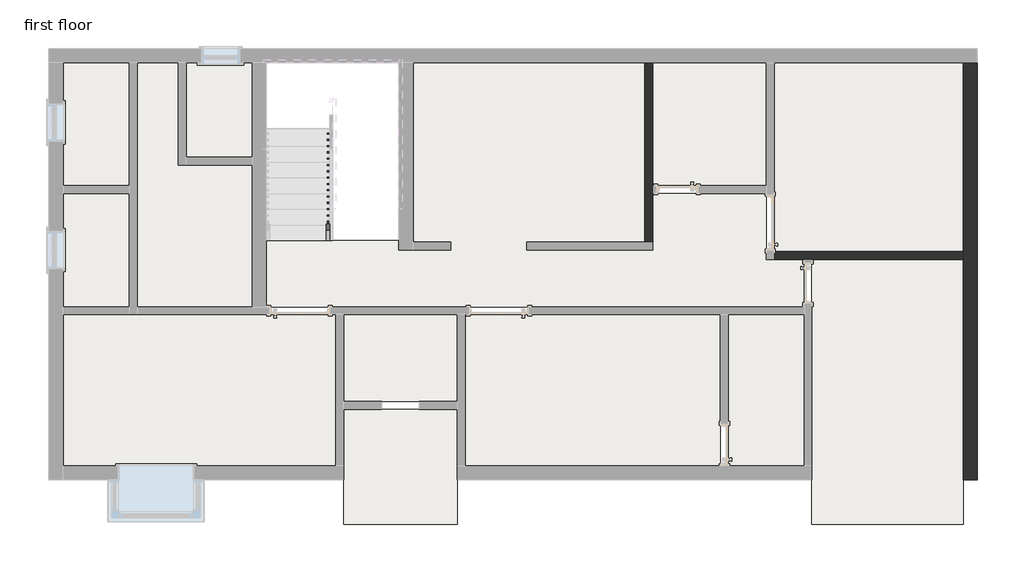
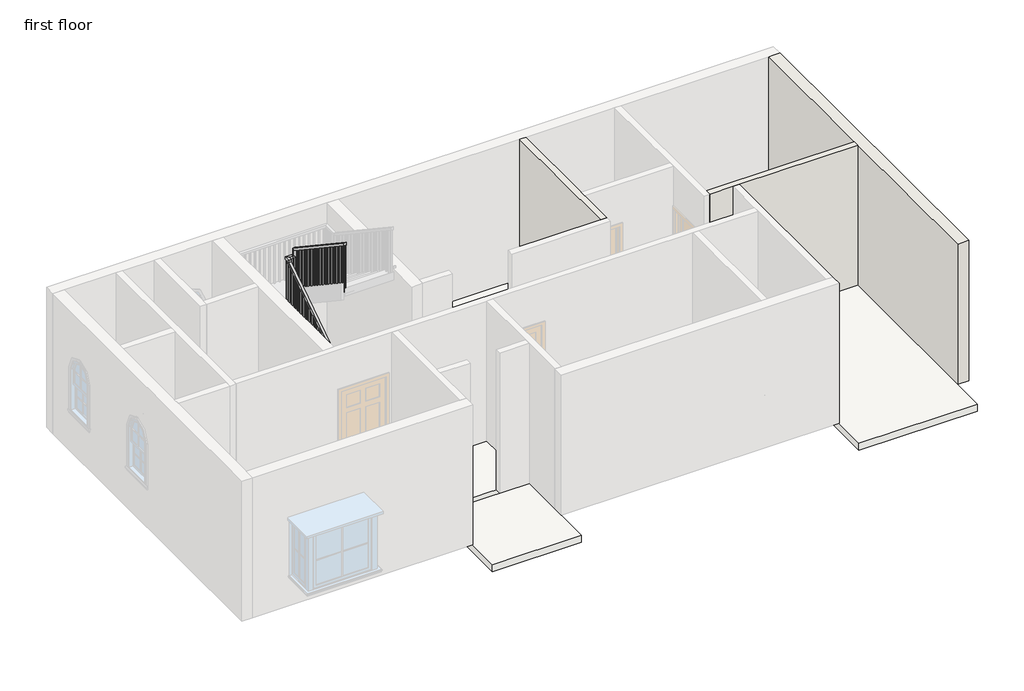
# One storey, part 2 of 3: 3 walls, 2 slabs, 1 railing.
"""IFC4 building model written with IfcOpenShell, lengths in millimetres."""

from ifc_helpers import new_model, si_unit, frame, origin, place, context, project, spatial, polyline, outline, extrude, faceted_brep, element, save

model = new_model("IFC4")

# Units and contexts
model_context = context("Model", 3, world=origin())
ifc_project = project(units=[si_unit("LENGTHUNIT", "METRE", prefix="MILLI")], contexts=[model_context])

# Site, building, storey
site = spatial("IfcSite", under=ifc_project)
building = spatial("IfcBuilding", under=site)
storey = spatial("IfcBuildingStorey", under=building, Name="first floor", Elevation=3352.8)

# Railing
placement = place(None, origin())
element("IfcRailing", 1, ObjectType="Handrail - Rectangular", at=placement, inside=storey, context=model_context, shape_type="SolidModel", body=[
    faceted_brep([(-8708.6672301, -3404.4302427, 4436.5333333), (-8708.6672301, -3404.4302427, 4375.4793317), (-8657.8672301, -3404.4302427, 4375.4793317), (-8657.8672301, -3404.4302427, 4436.5333333), (-8708.6672301, -1194.6302427, 5909.7333333), (-8708.6672301, -1143.8302427, 5882.5459984), (-8657.8672301, -1143.8302427, 5882.5459984), (-8657.8672301, -1194.6302427, 5909.7333333), (-8708.6672301, -1194.6302427, 5960.5333333), (-8708.6672301, -1143.8302427, 5909.7333333), (-8657.8672301, -1143.8302427, 5909.7333333), (-8657.8672301, -1194.6302427, 5960.5333333), (-8708.6672301, -1067.6302427, 5960.5333333), (-8708.6672301, -1067.6302427, 5909.7333333), (-8657.8672301, -1118.4302427, 5909.7333333), (-8657.8672301, -1118.4302427, 5960.5333333), (-8581.6672301, -1067.6302427, 5960.5333333), (-8581.6672301, -1067.6302427, 5909.7333333), (-8581.6672301, -1118.4302427, 5909.7333333), (-8581.6672301, -1118.4302427, 5960.5333333), (-8556.2672301, -1067.6302427, 5960.5333333), (-8556.2672301, -1118.4302427, 5960.5333333), (-8505.4672301, -1118.4302427, 5909.7333333), (-8505.4672301, -1067.6302427, 5909.7333333)], [[[0, 1, 2, 3]], [[1, 0, 4, 5]], [[2, 1, 5, 6]], [[3, 2, 6, 7]], [[0, 3, 7, 4]], [[5, 4, 8, 9]], [[6, 5, 9, 10]], [[7, 6, 10, 11]], [[4, 7, 11, 8]], [[9, 8, 12, 13]], [[10, 9, 13, 14]], [[11, 10, 14, 15]], [[8, 11, 15, 12]], [[13, 12, 16, 17]], [[14, 13, 17, 18]], [[15, 14, 18, 19]], [[12, 15, 19, 16]], [[20, 21, 22, 23]], [[17, 16, 20, 23]], [[18, 17, 23, 22]], [[19, 18, 22, 21]], [[16, 19, 21, 20]]]),
    faceted_brep([(-8556.2672301, -1067.6302427, 5960.5333333), (-8505.4672301, -1067.6302427, 5909.7333333), (-8505.4672301, -1118.4302427, 5909.7333333), (-8556.2672301, -1118.4302427, 5960.5333333), (-8556.2672301, -1067.6302427, 6096.0), (-8556.2672301, -1118.4302427, 6068.8126651), (-8505.4672301, -1118.4302427, 6068.8126651), (-8505.4672301, -1067.6302427, 6096.0)], [[[0, 1, 2, 3]], [[4, 5, 6, 7]], [[1, 0, 4, 7]], [[2, 1, 7, 6]], [[3, 2, 6, 5]], [[0, 3, 5, 4]]]),
    faceted_brep([(-8505.4672301, -1067.6302427, 6096.0), (-8505.4672301, -1118.4302427, 6068.8126651), (-8556.2672301, -1118.4302427, 6068.8126651), (-8556.2672301, -1067.6302427, 6096.0), (-8505.4672301, -2896.4302427, 7315.2), (-8556.2672301, -2896.4302427, 7315.2), (-8556.2672301, -2896.4302427, 7254.1459984), (-8505.4672301, -2896.4302427, 7254.1459984)], [[[0, 1, 2, 3]], [[4, 5, 6, 7]], [[1, 0, 4, 7]], [[2, 1, 7, 6]], [[3, 2, 6, 5]], [[0, 3, 5, 4]]]),
    extrude(outline(polyline([(-2829.7552427, 7209.6959984), (-2810.7052427, 7196.9959984), (-2810.7052427, 6231.4666667), (-2829.7552427, 6231.4666667), (-2829.7552427, 7209.6959984)])), frame((-8540.3922301, 0.0, 0.0), z_axis=(1.0, 0.0, 0.0), x_axis=(0.0, 1.0, 0.0)), (0.0, 0.0, 1.0), 19.05),
    extrude(outline(polyline([(-2728.1552427, 7141.9626651), (-2709.1052427, 7129.2626651), (-2709.1052427, 6231.4666667), (-2728.1552427, 6231.4666667), (-2728.1552427, 7141.9626651)])), frame((-8540.3922301, 0.0, 0.0), z_axis=(1.0, 0.0, 0.0), x_axis=(0.0, 1.0, 0.0)), (0.0, 0.0, 1.0), 19.05),
    extrude(outline(polyline([(-2626.5552427, 7074.2293317), (-2607.5052427, 7061.5293317), (-2607.5052427, 6062.1333333), (-2626.5552427, 6062.1333333), (-2626.5552427, 7074.2293317)])), frame((-8540.3922301, 0.0, 0.0), z_axis=(1.0, 0.0, 0.0), x_axis=(0.0, 1.0, 0.0)), (0.0, 0.0, 1.0), 19.05),
    extrude(outline(polyline([(-2524.9552427, 7006.4959984), (-2505.9052427, 6993.7959984), (-2505.9052427, 6062.1333333), (-2524.9552427, 6062.1333333), (-2524.9552427, 7006.4959984)])), frame((-8540.3922301, 0.0, 0.0), z_axis=(1.0, 0.0, 0.0), x_axis=(0.0, 1.0, 0.0)), (0.0, 0.0, 1.0), 19.05),
    extrude(outline(polyline([(-2423.3552427, 6938.7626651), (-2404.3052427, 6926.0626651), (-2404.3052427, 6062.1333333), (-2423.3552427, 6062.1333333), (-2423.3552427, 6938.7626651)])), frame((-8540.3922301, 0.0, 0.0), z_axis=(1.0, 0.0, 0.0), x_axis=(0.0, 1.0, 0.0)), (0.0, 0.0, 1.0), 19.05),
    extrude(outline(polyline([(-2321.7552427, 6871.0293317), (-2302.7052427, 6858.3293317), (-2302.7052427, 5892.8), (-2321.7552427, 5892.8), (-2321.7552427, 6871.0293317)])), frame((-8540.3922301, 0.0, 0.0), z_axis=(1.0, 0.0, 0.0), x_axis=(0.0, 1.0, 0.0)), (0.0, 0.0, 1.0), 19.05),
    extrude(outline(polyline([(-2220.1552427, 6803.2959984), (-2201.1052427, 6790.5959984), (-2201.1052427, 5892.8), (-2220.1552427, 5892.8), (-2220.1552427, 6803.2959984)])), frame((-8540.3922301, 0.0, 0.0), z_axis=(1.0, 0.0, 0.0), x_axis=(0.0, 1.0, 0.0)), (0.0, 0.0, 1.0), 19.05),
    extrude(outline(polyline([(-2118.5552427, 6735.5626651), (-2099.5052427, 6722.8626651), (-2099.5052427, 5723.4666667), (-2118.5552427, 5723.4666667), (-2118.5552427, 6735.5626651)])), frame((-8540.3922301, 0.0, 0.0), z_axis=(1.0, 0.0, 0.0), x_axis=(0.0, 1.0, 0.0)), (0.0, 0.0, 1.0), 19.05),
    extrude(outline(polyline([(-2016.9552427, 6667.8293317), (-1997.9052427, 6655.1293317), (-1997.9052427, 5723.4666667), (-2016.9552427, 5723.4666667), (-2016.9552427, 6667.8293317)])), frame((-8540.3922301, 0.0, 0.0), z_axis=(1.0, 0.0, 0.0), x_axis=(0.0, 1.0, 0.0)), (0.0, 0.0, 1.0), 19.05),
    extrude(outline(polyline([(-1915.3552427, 6600.0959984), (-1896.3052427, 6587.3959984), (-1896.3052427, 5723.4666667), (-1915.3552427, 5723.4666667), (-1915.3552427, 6600.0959984)])), frame((-8540.3922301, 0.0, 0.0), z_axis=(1.0, 0.0, 0.0), x_axis=(0.0, 1.0, 0.0)), (0.0, 0.0, 1.0), 19.05),
    extrude(outline(polyline([(-1813.7552427, 6532.3626651), (-1794.7052427, 6519.6626651), (-1794.7052427, 5554.1333333), (-1813.7552427, 5554.1333333), (-1813.7552427, 6532.3626651)])), frame((-8540.3922301, 0.0, 0.0), z_axis=(1.0, 0.0, 0.0), x_axis=(0.0, 1.0, 0.0)), (0.0, 0.0, 1.0), 19.05),
    extrude(outline(polyline([(-1712.1552427, 6464.6293317), (-1693.1052427, 6451.9293317), (-1693.1052427, 5554.1333333), (-1712.1552427, 5554.1333333), (-1712.1552427, 6464.6293317)])), frame((-8540.3922301, 0.0, 0.0), z_axis=(1.0, 0.0, 0.0), x_axis=(0.0, 1.0, 0.0)), (0.0, 0.0, 1.0), 19.05),
    extrude(outline(polyline([(-1610.5552427, 6396.8959984), (-1591.5052427, 6384.1959984), (-1591.5052427, 5384.8), (-1610.5552427, 5384.8), (-1610.5552427, 6396.8959984)])), frame((-8540.3922301, 0.0, 0.0), z_axis=(1.0, 0.0, 0.0), x_axis=(0.0, 1.0, 0.0)), (0.0, 0.0, 1.0), 19.05),
    extrude(outline(polyline([(-1508.9552427, 6329.1626651), (-1489.9052427, 6316.4626651), (-1489.9052427, 5384.8), (-1508.9552427, 5384.8), (-1508.9552427, 6329.1626651)])), frame((-8540.3922301, 0.0, 0.0), z_axis=(1.0, 0.0, 0.0), x_axis=(0.0, 1.0, 0.0)), (0.0, 0.0, 1.0), 19.05),
    extrude(outline(polyline([(-1407.3552427, 6261.4293317), (-1388.3052427, 6248.7293317), (-1388.3052427, 5384.8), (-1407.3552427, 5384.8), (-1407.3552427, 6261.4293317)])), frame((-8540.3922301, 0.0, 0.0), z_axis=(1.0, 0.0, 0.0), x_axis=(0.0, 1.0, 0.0)), (0.0, 0.0, 1.0), 19.05),
    extrude(outline(polyline([(-1305.7552427, 6193.6959984), (-1286.7052427, 6180.9959984), (-1286.7052427, 5215.4666667), (-1305.7552427, 5215.4666667), (-1305.7552427, 6193.6959984)])), frame((-8540.3922301, 0.0, 0.0), z_axis=(1.0, 0.0, 0.0), x_axis=(0.0, 1.0, 0.0)), (0.0, 0.0, 1.0), 19.05),
    extrude(outline(polyline([(-1204.1552427, 6125.9626651), (-1185.1052427, 6113.2626651), (-1185.1052427, 5215.4666667), (-1204.1552427, 5215.4666667), (-1204.1552427, 6125.9626651)])), frame((-8540.3922301, 0.0, 0.0), z_axis=(1.0, 0.0, 0.0), x_axis=(0.0, 1.0, 0.0)), (0.0, 0.0, 1.0), 19.05),
    extrude(outline(polyline([(-8591.1922301, -1102.5552427), (-8591.1922301, -1083.5052427), (-8572.1422301, -1083.5052427), (-8572.1422301, -1102.5552427), (-8591.1922301, -1102.5552427)])), frame((0.0, 0.0, 5046.1333333), z_axis=(0.0, 0.0, 1.0), x_axis=(1.0, 0.0, 0.0)), (0.0, 0.0, 1.0), 863.6),
    extrude(outline(polyline([(-8673.7422301, -1178.7552427), (-8692.7922301, -1178.7552427), (-8692.7922301, -1159.7052427), (-8673.7422301, -1159.7052427), (-8673.7422301, -1178.7552427)])), frame((0.0, 0.0, 4876.8), z_axis=(0.0, 0.0, 1.0), x_axis=(1.0, 0.0, 0.0)), (0.0, 0.0, 1.0), 1032.9333333),
    extrude(outline(polyline([(-1280.3552427, 5791.5293317), (-1261.3052427, 5804.2293317), (-1261.3052427, 4876.8), (-1280.3552427, 4876.8), (-1280.3552427, 5791.5293317)])), frame((-8692.7922301, 0.0, 0.0), z_axis=(1.0, 0.0, 0.0), x_axis=(0.0, 1.0, 0.0)), (0.0, 0.0, 1.0), 19.05),
    extrude(outline(polyline([(-1381.9552427, 5723.7959984), (-1362.9052427, 5736.4959984), (-1362.9052427, 4876.8), (-1381.9552427, 4876.8), (-1381.9552427, 5723.7959984)])), frame((-8692.7922301, 0.0, 0.0), z_axis=(1.0, 0.0, 0.0), x_axis=(0.0, 1.0, 0.0)), (0.0, 0.0, 1.0), 19.05),
    extrude(outline(polyline([(-1483.5552427, 5656.0626651), (-1464.5052427, 5668.7626651), (-1464.5052427, 4707.4666667), (-1483.5552427, 4707.4666667), (-1483.5552427, 5656.0626651)])), frame((-8692.7922301, 0.0, 0.0), z_axis=(1.0, 0.0, 0.0), x_axis=(0.0, 1.0, 0.0)), (0.0, 0.0, 1.0), 19.05),
    extrude(outline(polyline([(-1585.1552427, 5588.3293317), (-1566.1052427, 5601.0293317), (-1566.1052427, 4707.4666667), (-1585.1552427, 4707.4666667), (-1585.1552427, 5588.3293317)])), frame((-8692.7922301, 0.0, 0.0), z_axis=(1.0, 0.0, 0.0), x_axis=(0.0, 1.0, 0.0)), (0.0, 0.0, 1.0), 19.05),
    extrude(outline(polyline([(-1686.7552427, 5520.5959984), (-1667.7052427, 5533.2959984), (-1667.7052427, 4538.1333333), (-1686.7552427, 4538.1333333), (-1686.7552427, 5520.5959984)])), frame((-8692.7922301, 0.0, 0.0), z_axis=(1.0, 0.0, 0.0), x_axis=(0.0, 1.0, 0.0)), (0.0, 0.0, 1.0), 19.05),
    extrude(outline(polyline([(-1788.3552427, 5452.8626651), (-1769.3052427, 5465.5626651), (-1769.3052427, 4538.1333333), (-1788.3552427, 4538.1333333), (-1788.3552427, 5452.8626651)])), frame((-8692.7922301, 0.0, 0.0), z_axis=(1.0, 0.0, 0.0), x_axis=(0.0, 1.0, 0.0)), (0.0, 0.0, 1.0), 19.05),
    extrude(outline(polyline([(-1889.9552427, 5385.1293317), (-1870.9052427, 5397.8293317), (-1870.9052427, 4538.1333333), (-1889.9552427, 4538.1333333), (-1889.9552427, 5385.1293317)])), frame((-8692.7922301, 0.0, 0.0), z_axis=(1.0, 0.0, 0.0), x_axis=(0.0, 1.0, 0.0)), (0.0, 0.0, 1.0), 19.05),
    extrude(outline(polyline([(-1991.5552427, 5317.3959984), (-1972.5052427, 5330.0959984), (-1972.5052427, 4368.8), (-1991.5552427, 4368.8), (-1991.5552427, 5317.3959984)])), frame((-8692.7922301, 0.0, 0.0), z_axis=(1.0, 0.0, 0.0), x_axis=(0.0, 1.0, 0.0)), (0.0, 0.0, 1.0), 19.05),
    extrude(outline(polyline([(-2093.1552427, 5249.6626651), (-2074.1052427, 5262.3626651), (-2074.1052427, 4368.8), (-2093.1552427, 4368.8), (-2093.1552427, 5249.6626651)])), frame((-8692.7922301, 0.0, 0.0), z_axis=(1.0, 0.0, 0.0), x_axis=(0.0, 1.0, 0.0)), (0.0, 0.0, 1.0), 19.05),
    extrude(outline(polyline([(-2194.7552427, 5181.9293317), (-2175.7052427, 5194.6293317), (-2175.7052427, 4199.4666667), (-2194.7552427, 4199.4666667), (-2194.7552427, 5181.9293317)])), frame((-8692.7922301, 0.0, 0.0), z_axis=(1.0, 0.0, 0.0), x_axis=(0.0, 1.0, 0.0)), (0.0, 0.0, 1.0), 19.05),
    extrude(outline(polyline([(-2296.3552427, 5114.1959984), (-2277.3052427, 5126.8959984), (-2277.3052427, 4199.4666667), (-2296.3552427, 4199.4666667), (-2296.3552427, 5114.1959984)])), frame((-8692.7922301, 0.0, 0.0), z_axis=(1.0, 0.0, 0.0), x_axis=(0.0, 1.0, 0.0)), (0.0, 0.0, 1.0), 19.05),
    extrude(outline(polyline([(-2397.9552427, 5046.4626651), (-2378.9052427, 5059.1626651), (-2378.9052427, 4199.4666667), (-2397.9552427, 4199.4666667), (-2397.9552427, 5046.4626651)])), frame((-8692.7922301, 0.0, 0.0), z_axis=(1.0, 0.0, 0.0), x_axis=(0.0, 1.0, 0.0)), (0.0, 0.0, 1.0), 19.05),
    extrude(outline(polyline([(-2499.5552427, 4978.7293317), (-2480.5052427, 4991.4293317), (-2480.5052427, 4030.1333333), (-2499.5552427, 4030.1333333), (-2499.5552427, 4978.7293317)])), frame((-8692.7922301, 0.0, 0.0), z_axis=(1.0, 0.0, 0.0), x_axis=(0.0, 1.0, 0.0)), (0.0, 0.0, 1.0), 19.05),
    extrude(outline(polyline([(-2601.1552427, 4910.9959984), (-2582.1052427, 4923.6959984), (-2582.1052427, 4030.1333333), (-2601.1552427, 4030.1333333), (-2601.1552427, 4910.9959984)])), frame((-8692.7922301, 0.0, 0.0), z_axis=(1.0, 0.0, 0.0), x_axis=(0.0, 1.0, 0.0)), (0.0, 0.0, 1.0), 19.05),
    extrude(outline(polyline([(-2702.7552427, 4843.2626651), (-2683.7052427, 4855.9626651), (-2683.7052427, 3860.8), (-2702.7552427, 3860.8), (-2702.7552427, 4843.2626651)])), frame((-8692.7922301, 0.0, 0.0), z_axis=(1.0, 0.0, 0.0), x_axis=(0.0, 1.0, 0.0)), (0.0, 0.0, 1.0), 19.05),
    extrude(outline(polyline([(-2804.3552427, 4775.5293317), (-2785.3052427, 4788.2293317), (-2785.3052427, 3860.8), (-2804.3552427, 3860.8), (-2804.3552427, 4775.5293317)])), frame((-8692.7922301, 0.0, 0.0), z_axis=(1.0, 0.0, 0.0), x_axis=(0.0, 1.0, 0.0)), (0.0, 0.0, 1.0), 19.05),
    extrude(outline(polyline([(-2905.9552427, 4707.7959984), (-2886.9052427, 4720.4959984), (-2886.9052427, 3860.8), (-2905.9552427, 3860.8), (-2905.9552427, 4707.7959984)])), frame((-8692.7922301, 0.0, 0.0), z_axis=(1.0, 0.0, 0.0), x_axis=(0.0, 1.0, 0.0)), (0.0, 0.0, 1.0), 19.05),
    extrude(outline(polyline([(-3007.5552427, 4640.0626651), (-2988.5052427, 4652.7626651), (-2988.5052427, 3691.4666667), (-3007.5552427, 3691.4666667), (-3007.5552427, 4640.0626651)])), frame((-8692.7922301, 0.0, 0.0), z_axis=(1.0, 0.0, 0.0), x_axis=(0.0, 1.0, 0.0)), (0.0, 0.0, 1.0), 19.05),
    extrude(outline(polyline([(-3109.1552427, 4572.3293317), (-3090.1052427, 4585.0293317), (-3090.1052427, 3691.4666667), (-3109.1552427, 3691.4666667), (-3109.1552427, 4572.3293317)])), frame((-8692.7922301, 0.0, 0.0), z_axis=(1.0, 0.0, 0.0), x_axis=(0.0, 1.0, 0.0)), (0.0, 0.0, 1.0), 19.05),
    extrude(outline(polyline([(-3210.7552427, 4504.5959984), (-3191.7052427, 4517.2959984), (-3191.7052427, 3522.1333333), (-3210.7552427, 3522.1333333), (-3210.7552427, 4504.5959984)])), frame((-8692.7922301, 0.0, 0.0), z_axis=(1.0, 0.0, 0.0), x_axis=(0.0, 1.0, 0.0)), (0.0, 0.0, 1.0), 19.05),
    extrude(outline(polyline([(-3312.3552427, 4436.8626651), (-3293.3052427, 4449.5626651), (-3293.3052427, 3522.1333333), (-3312.3552427, 3522.1333333), (-3312.3552427, 4436.8626651)])), frame((-8692.7922301, 0.0, 0.0), z_axis=(1.0, 0.0, 0.0), x_axis=(0.0, 1.0, 0.0)), (0.0, 0.0, 1.0), 19.05),
    extrude(outline(polyline([(-8540.3922301, -1102.5552427), (-8540.3922301, -1083.5052427), (-8521.3422301, -1083.5052427), (-8521.3422301, -1102.5552427), (-8540.3922301, -1102.5552427)])), frame((0.0, 0.0, 5046.1333333), z_axis=(0.0, 0.0, 1.0), x_axis=(1.0, 0.0, 0.0)), (0.0, 0.0, 1.0), 863.6),
    extrude(outline(polyline([(-8673.7422301, -1102.5552427), (-8692.7922301, -1102.5552427), (-8692.7922301, -1083.5052427), (-8673.7422301, -1083.5052427), (-8673.7422301, -1102.5552427)])), frame((0.0, 0.0, 5046.1333333), z_axis=(0.0, 0.0, 1.0), x_axis=(1.0, 0.0, 0.0)), (0.0, 0.0, 1.0), 863.6),
    extrude(outline(polyline([(-2896.4302427, 7254.1459984), (-2877.3802427, 7241.4459984), (-2877.3802427, 6231.4666667), (-2896.4302427, 6231.4666667), (-2896.4302427, 7254.1459984)])), frame((-8540.3922301, 0.0, 0.0), z_axis=(1.0, 0.0, 0.0), x_axis=(0.0, 1.0, 0.0)), (0.0, 0.0, 1.0), 19.05),
    extrude(outline(polyline([(-3404.4302427, 4375.4793317), (-3385.3802427, 4388.1793317), (-3385.3802427, 3522.1333333), (-3404.4302427, 3522.1333333), (-3404.4302427, 4375.4793317)])), frame((-8692.7922301, 0.0, 0.0), z_axis=(1.0, 0.0, 0.0), x_axis=(0.0, 1.0, 0.0)), (0.0, 0.0, 1.0), 19.05),
])

# Slabs
element("IfcSlab", 2, ObjectType="FIRST FLOOR FLOORING 6\"", at=placement, inside=storey, context=model_context, shape_type="SweptSolid", body=[
    extrude(outline(polyline([(1552.9327699, -534.2302427), (1552.9327699, -3582.2302427), (-1495.0672301, -3582.2302427), (-1495.0672301, -534.2302427), (1552.9327699, -534.2302427)])), frame((0.0, 0.0, 3200.4), z_axis=(0.0, 0.0, 1.0), x_axis=(1.0, 0.0, 0.0)), (0.0, 0.0, 1.0), 152.4),
    extrude(outline(polyline([(1552.9327699, -3709.2302427), (1552.9327699, -7976.4302427), (-885.4672301, -7976.4302427), (-885.4672301, -3709.2302427), (1552.9327699, -3709.2302427)])), frame((0.0, 0.0, 3200.4), z_axis=(0.0, 0.0, 1.0), x_axis=(1.0, 0.0, 0.0)), (0.0, 0.0, 1.0), 152.4),
    extrude(outline(polyline([(-1622.0672301, -534.2302427), (-1622.0672301, -2515.4302427), (-3450.8672301, -2515.4302427), (-3450.8672301, -534.2302427), (-1622.0672301, -534.2302427)])), frame((0.0, 0.0, 3200.4), z_axis=(0.0, 0.0, 1.0), x_axis=(1.0, 0.0, 0.0)), (0.0, 0.0, 1.0), 152.4),
    extrude(outline(polyline([(-11883.6672301, -534.2302427), (-11883.6672301, -2515.4302427), (-12950.4672301, -2515.4302427), (-12950.4672301, -534.2302427), (-11883.6672301, -534.2302427)])), frame((0.0, 0.0, 3200.4), z_axis=(0.0, 0.0, 1.0), x_axis=(1.0, 0.0, 0.0)), (0.0, 0.0, 1.0), 152.4),
    extrude(outline(polyline([(-9902.4672301, -534.2302427), (-9902.4672301, -2058.2302427), (-10969.2672301, -2058.2302427), (-10969.2672301, -534.2302427), (-9902.4672301, -534.2302427)])), frame((0.0, 0.0, 3200.4), z_axis=(0.0, 0.0, 1.0), x_axis=(1.0, 0.0, 0.0)), (0.0, 0.0, 1.0), 152.4),
    extrude(outline(polyline([(-8556.2672301, -4598.2302427), (-8556.2672301, -7036.6302427), (-12950.4672301, -7036.6302427), (-12950.4672301, -4598.2302427), (-8556.2672301, -4598.2302427)])), frame((0.0, 0.0, 3200.4), z_axis=(0.0, 0.0, 1.0), x_axis=(1.0, 0.0, 0.0)), (0.0, 0.0, 1.0), 152.4),
    extrude(outline(polyline([(-6600.4672301, -4598.2302427), (-6600.4672301, -5995.2302427), (-8429.2672301, -5995.2302427), (-8429.2672301, -4598.2302427), (-6600.4672301, -4598.2302427)])), frame((0.0, 0.0, 3200.4), z_axis=(0.0, 0.0, 1.0), x_axis=(1.0, 0.0, 0.0)), (0.0, 0.0, 1.0), 152.4),
    extrude(outline(polyline([(-6600.4672301, -6122.2302427), (-6600.4672301, -7976.4302427), (-8429.2672301, -7976.4302427), (-8429.2672301, -6122.2302427), (-6600.4672301, -6122.2302427)])), frame((0.0, 0.0, 3200.4), z_axis=(0.0, 0.0, 1.0), x_axis=(1.0, 0.0, 0.0)), (0.0, 0.0, 1.0), 152.4),
    extrude(outline(polyline([(-9902.4672301, -4471.2302427), (-11756.6672301, -4471.2302427), (-11756.6672301, -534.2302427), (-11096.2672301, -534.2302427), (-11096.2672301, -2185.2302427), (-9902.4672301, -2185.2302427), (-9902.4672301, -4471.2302427)])), frame((0.0, 0.0, 3200.4), z_axis=(0.0, 0.0, 1.0), x_axis=(1.0, 0.0, 0.0)), (0.0, 0.0, 1.0), 152.4),
    extrude(outline(polyline([(-1012.4672301, -4471.2302427), (-9673.8672301, -4471.2302427), (-9673.8672301, -3404.4302427), (-7540.2672301, -3404.4302427), (-7540.2672301, -3556.8302427), (-7425.9672301, -3556.8302427), (-6702.0672301, -3556.8302427), (-6702.0672301, -3429.8302427), (-7311.6672301, -3429.8302427), (-7311.6672301, -534.2302427), (-3577.8672301, -534.2302427), (-3577.8672301, -3429.8302427), (-5482.8672301, -3429.8302427), (-5482.8672301, -3556.8302427), (-3450.8672301, -3556.8302427), (-3450.8672301, -2642.4302427), (-1622.0672301, -2642.4302427), (-1622.0672301, -3709.2302427), (-1012.4672301, -3709.2302427), (-1012.4672301, -4471.2302427)])), frame((0.0, 0.0, 3200.4), z_axis=(0.0, 0.0, 1.0), x_axis=(1.0, 0.0, 0.0)), (0.0, 0.0, 1.0), 152.4),
    extrude(outline(polyline([(-2358.6672301, -4598.2302427), (-2358.6672301, -7036.6302427), (-6473.4672301, -7036.6302427), (-6473.4672301, -4598.2302427), (-2358.6672301, -4598.2302427)])), frame((0.0, 0.0, 3200.4), z_axis=(0.0, 0.0, 1.0), x_axis=(1.0, 0.0, 0.0)), (0.0, 0.0, 1.0), 152.4),
    extrude(outline(polyline([(-1012.4672301, -4598.2302427), (-1012.4672301, -7036.6302427), (-2231.6672301, -7036.6302427), (-2231.6672301, -4598.2302427), (-1012.4672301, -4598.2302427)])), frame((0.0, 0.0, 3200.4), z_axis=(0.0, 0.0, 1.0), x_axis=(1.0, 0.0, 0.0)), (0.0, 0.0, 1.0), 152.4),
    extrude(outline(polyline([(-11883.6672301, -2642.4302427), (-11883.6672301, -4471.2302427), (-12950.4672301, -4471.2302427), (-12950.4672301, -2642.4302427), (-11883.6672301, -2642.4302427)])), frame((0.0, 0.0, 3200.4), z_axis=(0.0, 0.0, 1.0), x_axis=(1.0, 0.0, 0.0)), (0.0, 0.0, 1.0), 152.4),
])
element("IfcSlab", 3, ObjectType="FIRST FLOOR FLOORING 6\"", at=placement, inside=storey, context=model_context, shape_type="SweptSolid", body=[
    extrude(outline(polyline([(-11883.6672301, -2642.4302427), (-11883.6672301, -4471.2302427), (-12950.4672301, -4471.2302427), (-12950.4672301, -2642.4302427), (-11883.6672301, -2642.4302427)])), frame((0.0, 0.0, 3200.4), z_axis=(0.0, 0.0, 1.0), x_axis=(1.0, 0.0, 0.0)), (0.0, 0.0, 1.0), 152.4),
    extrude(outline(polyline([(-9902.4672301, -4471.2302427), (-11756.6672301, -4471.2302427), (-11756.6672301, -534.2302427), (-11096.2672301, -534.2302427), (-11096.2672301, -2185.2302427), (-9902.4672301, -2185.2302427), (-9902.4672301, -4471.2302427)])), frame((0.0, 0.0, 3200.4), z_axis=(0.0, 0.0, 1.0), x_axis=(1.0, 0.0, 0.0)), (0.0, 0.0, 1.0), 152.4),
])

# Walls
element("IfcWall", 4, ObjectType="INNER WALL 5\"", at=placement, inside=storey, context=model_context, shape_type="Brep", body=[
    faceted_brep([(-3450.8672301, -3429.8302427, 3352.8), (-3450.8672301, -2642.4302427, 3352.8), (-3450.8672301, -2515.4302427, 3352.8), (-3450.8672301, -534.2302427, 3352.8), (-3450.8672301, -534.2302427, 6400.8), (-3450.8672301, -2515.4302427, 6400.8), (-3450.8672301, -2642.4302427, 6400.8), (-3450.8672301, -3429.8302427, 6400.8), (-3577.8672301, -3429.8302427, 3352.8), (-3577.8672301, -3429.8302427, 6400.8), (-3577.8672301, -534.2302427, 6400.8), (-3577.8672301, -534.2302427, 3352.8)], [[[0, 1, 2, 3, 4, 5, 6, 7]], [[8, 9, 10, 11]], [[3, 2, 1, 0, 8, 11]], [[7, 6, 5, 4, 10, 9]], [[0, 7, 9, 8]], [[4, 3, 11, 10]]]),
])
element("IfcWall", 5, ObjectType="INNER WALL 5\"", at=placement, inside=storey, context=model_context, shape_type="Brep", body=[
    faceted_brep([(-1495.0672301, -3709.2302427, 3352.8), (-1012.4672301, -3709.2302427, 3352.8), (-885.4672301, -3709.2302427, 3352.8), (1552.9327699, -3709.2302427, 3352.8), (1552.9327699, -3709.2302427, 6400.8), (-885.4672301, -3709.2302427, 6400.8), (-1012.4672301, -3709.2302427, 6400.8), (-1495.0672301, -3709.2302427, 6400.8), (-1495.0672301, -3582.2302427, 3352.8), (-1495.0672301, -3582.2302427, 6400.8), (1552.9327699, -3582.2302427, 6400.8), (1552.9327699, -3582.2302427, 3352.8)], [[[0, 1, 2, 3, 4, 5, 6, 7]], [[8, 9, 10, 11]], [[3, 2, 1, 0, 8, 11]], [[7, 6, 5, 4, 10, 9]], [[0, 7, 9, 8]], [[4, 3, 11, 10]]]),
])
element("IfcWall", 6, ObjectType="OUTER WALL 9\"", at=placement, inside=storey, context=model_context, shape_type="Brep", body=[
    faceted_brep([(1781.5327699, -7265.2302427, 3352.8), (1781.5327699, -534.2302427, 3352.8), (1781.5327699, -534.2302427, 6400.8), (1781.5327699, -7265.2302427, 6400.8), (1552.9327699, -7265.2302427, 3352.8), (1552.9327699, -7265.2302427, 6400.8), (1552.9327699, -3709.2302427, 6400.8), (1552.9327699, -3582.2302427, 6400.8), (1552.9327699, -534.2302427, 6400.8), (1552.9327699, -534.2302427, 3352.8), (1552.9327699, -3582.2302427, 3352.8), (1552.9327699, -3709.2302427, 3352.8)], [[[0, 1, 2, 3]], [[4, 5, 6, 7, 8, 9, 10, 11]], [[1, 0, 4, 11, 10, 9]], [[3, 2, 8, 7, 6, 5]], [[0, 3, 5, 4]], [[2, 1, 9, 8]]]),
])

save(model, "model.ifc")

# Revit data of these elements
# Type "Handrail - Rectangular"
#   Assembly Code = "C2010400"
#   built-in parameter 1008612 = 0.0416667 (stored number, unit not read)
#   built-in parameter 1008611 = 0.0416667 (stored number, unit not read)
#   built-in parameter 1008609 = 0.333333 (stored number, unit not read)
#   built-in parameter 1008604 = 0.166667 (stored number, unit not read)
#   built-in parameter 1008603 = 0.166667 (stored number, unit not read)
#   Railing Height = 3' - 0"
#   built-in parameter 1008630 = 2
#   built-in parameter 1008610 = 2
#   built-in parameter 1008618 = Baluster - Square : 3/4"
# Type "FIRST FLOOR FLOORING 6\""
#   Assembly Code = "B1010"
#   Function = 0
#   Layers, outside or top first: 0' - 6" "MARBLE FLOORING 6\"" (function 1)
# Type "INNER WALL 5\""
#   Assembly Code = "B2010"
#   Layers, outside or top first: 0' - 5" "WARM BEIGE COLOUR" (function 1)
# Type "OUTER WALL 9\""
#   Assembly Code = "B2010"
#   Layers, outside or top first: 0' - 9" "WARM BEIGE COLOUR" (function 1)
# Element 1 (IfcRailing, "Handrail - Rectangular")
#   Phase Created = New Construction
# Elements 2, 3 (IfcSlab, "FIRST FLOOR FLOORING 6\"")
#   Height Offset From Level = 0' - 0"
#   Phase Created = New Construction
#   Materials on its faces: "MARBLE FLOORING 6\""
# Elements 4, 5 (IfcWall, "INNER WALL 5\"")
#   Top Offset = 0' - 0"
#   Base Offset = 0' - 0"
#   wall height = 10' - 0"
#   Phase Created = New Construction
#   Base Constraint = first floor
#   Top Constraint = TOP OF THE BUILDING
#   Materials on its faces: "WARM BEIGE COLOUR"
# Element 6 (IfcWall, "OUTER WALL 9\"")
#   Top Offset = 0' - 0"
#   Base Offset = 0' - 0"
#   wall height = 10' - 0"
#   Phase Created = New Construction
#   Base Constraint = first floor
#   Top Constraint = TOP OF THE BUILDING
#   Materials on its faces: "WARM BEIGE COLOUR"
# Materials
#   "MARBLE FLOORING 6\"": class "Generic", colour RGB 120 120 120, transparency 0, Cost = 0
#   "WARM BEIGE COLOUR": class "Generic", colour RGB 120 120 120, transparency 0, Cost = 0
